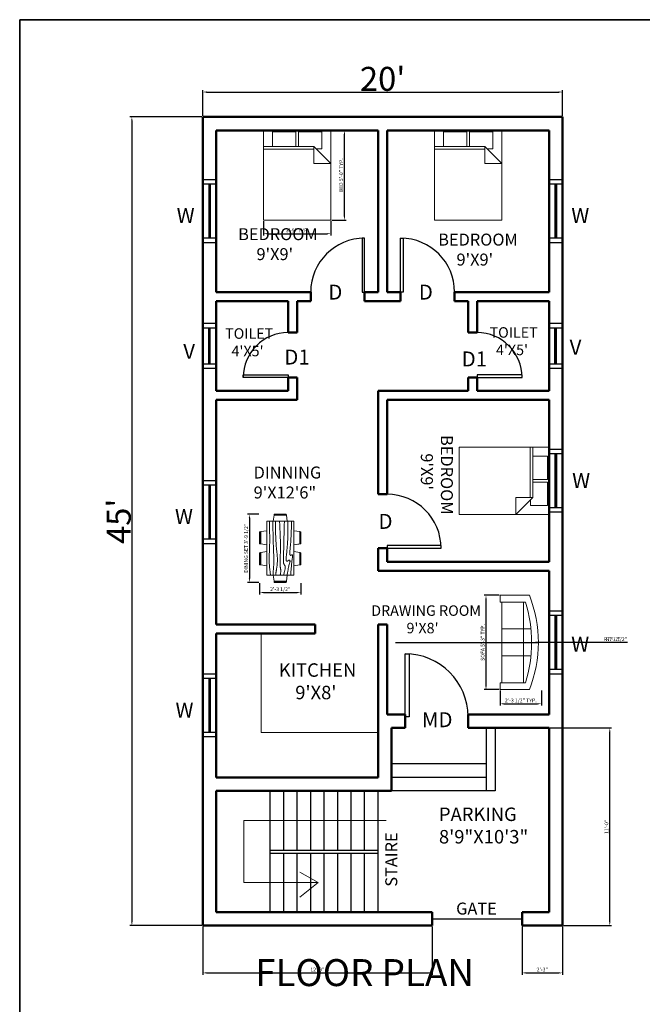
# Model space of a CAD drawing. Units: inches. Extents: x 2150 to 10686, y 1035 to 5077.
# Tile 11 of 12: x 9808 to 10224, y 1433 to 2091. Entities that reach past the tile are written whole.
import ezdxf

# ---------------------------------------------------------------- set-up
doc = ezdxf.new("R2010")
doc.units = ezdxf.units.IN
for name, color, linetype, lineweight in [('A-ANNO-DIMS', 2, 'Continuous', 18), ('A-ANNO-IDEN', 2, 'Continuous', 18), ('A-ANNO-SYMB', 3, 'Continuous', 18), ('A-ANNO-TITL', 3, 'Continuous', 35), ('A-ANNO-TTLB', 7, 'Continuous', 35), ('A-AREA-IDEN', 7, 'Continuous', 18), ('A-DOOR', 4, 'Continuous', 25), ('A-FLOR-FIXT', 9, 'Continuous', 18), ('A-FLOR-STRS', 4, 'Continuous', 25), ('A-FURN', 8, 'Continuous', 18), ('A-GLAZ', 30, 'Continuous', 25), ('A-WALL', 18, 'Continuous', 50)]:
    doc.layers.add(name, color=color, linetype=linetype, lineweight=lineweight)
doc.styles.get("Standard").update_dxf_attribs({"font": 'arial.ttf'})
doc.dimstyles.new('ISO-25', dxfattribs={"dimtxt": 2.5, "dimasz": 2.5, "dimexe": 1.25, "dimexo": 0.625, "dimtad": 1, "dimdec": 0, "dimlunit": 3, "dimtxsty": 'Standard', "dimcen": 2.5, "dimadec": 0, "dimazin": 0, "dimtfac": 1, "dimtdec": 0, "dimtmove": 0, "dimatfit": 3, "dimfxl": 1, "dimarcsym": 0})

# ---------------------------------------------------------------- blocks, each defined once
blk = doc.blocks.new('*U8')
for p, q in [((0, 0), (0, -6)), ((36, 0), (36, -6))]:
    blk.add_line(p, q)
blk.add_lwpolyline([(0, 0), (0, 36), (1.75, 36), (1.75, 0)], close=True)
blk.add_arc((0, 0), 36, 0, 90)
blk = doc.blocks.new('*U9')
for p, q in [((0, 0), (0, -6)), ((-36, 0), (-36, -6))]:
    blk.add_line(p, q)
blk.add_lwpolyline([(0, 0), (0, 36), (-1.75, 36), (-1.75, 0)], close=True)
blk.add_arc((0, 0), 36, 90, 180)
blk = doc.blocks.new('*U10')
for p, q in [((-30, 0), (-30, -6)), ((0, 0), (0, -6))]:
    blk.add_line(p, q)
blk.add_lwpolyline([(0, 0), (0, 30), (-1.75, 30), (-1.75, 0)], close=True)
blk.add_arc((0, 0), 30, 90, 180)
blk = doc.blocks.new('*U14')
for p, q in [((-30, 0), (-30, 6)), ((0, 0), (0, 6))]:
    blk.add_line(p, q)
blk.add_lwpolyline([(0, 0), (0, -30), (-1.75, -30), (-1.75, 0)], close=True)
blk.add_arc((0, 0), 30, 180, 270)
blk = doc.blocks.new('*U15')
for p, q in [((0, 0), (0, -5)), ((28, 0), (28, -5))]:
    blk.add_line(p, q)
blk.add_lwpolyline([(0, 0), (0, 28), (1.75, 28), (1.75, 0)], close=True)
blk.add_arc((0, 0), 28, 0, 90)
blk = doc.blocks.new('Bed - Queen')
for p, q in [((0, -80.00003), (0, 0)), ((0, 0), (59.99999, 0)), ((59.99999, 0), (59.99999, -80.00003)), ((7.99999, -1.2), (28.79998, -1.2)), ((7.99999, -14.4), (7.99999, -1.2)), ((28.79998, -1.2), (28.79998, -14.4)), ((31.19999, -1.2), (51.99999, -1.2)), ((31.19999, -14.4), (31.19999, -1.2)), ((51.99999, -1.2), (51.99999, -16.4)), ((0, -14.4), (44.8, -14.4)), ((44.8, -16.8), (0, -16.8)), ((59.99999, -29.6), (44.8, -14.4)), ((44.8, -14.4), (44.8, -29.6)), ((51.99999, -16.4), (46.79936, -16.4)), ((44.8, -29.6), (59.99999, -29.6)), ((59.99999, -80.00003), (0, -80.00003))]:
    blk.add_line(p, q)
blk = doc.blocks.new('Sofa - Roundback 7 ft.')
for p, q in [((-12.00002, -32.4421), (-12.00003, -6.5971)), ((11.99997, -32.4421), (11.99998, -6.5971)), ((-36.000027, -34), (-36.000027, -11.4696)), ((-35.999844, -13.3819), (35.9998, -13.3819)), ((35.99998, -34), (35.99998, -11.4696)), ((-36.000027, -32.4421), (35.99998, -32.4421))]:
    blk.add_line(p, q)
for points in [[(-36.000027, -34), (-42.000027, -34), (-42.000027, -8)], [(41.99998, -8), (41.99998, -34), (35.99998, -34)]]:
    blk.add_lwpolyline(points)
for centre, radius, start, end in [((0, -114.25), 114.25, 68.43141, 111.5686), ((-0.00001, -127.1968), 121.1968, 72.72033, 107.2797)]:
    blk.add_arc(centre, radius, start, end)
blk = doc.blocks.new('Dining Set - 36 x 72 in.')
for p, q in [((-22, 27.5), (-22.1562, 26.50042)), ((-5.8416, 26.5), (-22.1534, 26.5)), ((-22, 27.5), (-6, 27.5)), ((-5.14035, 21.99844), (-6, 27.5)), ((6, 27.5), (5.8438, 26.50042)), ((22.1584, 26.5), (5.8466, 26.5)), ((6, 27.5), (22, 27.5)), ((22.1563, 26.49966), (22, 27.5)), ((36, 18), (-36, 18)), ((-36, 18), (-36, -18)), ((-22.2343, 26.00059), (-23.4847, 17.99762)), ((-22.2304, 26), (-5.7608, 26)), ((-4.5152, 17.99762), (-5.7655, 25.99926)), ((5.7657, 26.00059), (4.5153, 17.99762)), ((5.7696, 26), (22.2392, 26)), ((23.4848, 17.99762), (22.2345, 25.99926)), ((36, -18), (36, 18)), ((-45.5, 8), (-44.5004, 8.15617)), ((-45.5, 8), (-45.5, -8)), ((-44.5, -8.15843), (-44.5, 8.15338)), ((-44.0006, 8.23428), (-35.9976, 9.48474)), ((-44, 8.23041), (-44, -8.23915)), ((44.0006, 8.23428), (35.9976, 9.48474)), ((44, 8.23041), (44, -8.23915)), ((44.5, -8.15843), (44.5, 8.15338)), ((45.5, 8), (44.5005, 8.15617)), ((45.5, 8), (45.5, -8)), ((-44.4997, -8.15631), (-45.5, -8)), ((-35.9976, -9.48476), (-43.9993, -8.2345)), ((35.9976, -9.48476), (43.9993, -8.2345)), ((44.4997, -8.15631), (45.5, -8)), ((-36, -18), (36, -18)), ((-22.2343, -26.0006), (-23.4847, -17.99762)), ((-22.2304, -26), (-5.7608, -26)), ((-4.5152, -17.99762), (-5.7655, -25.99928)), ((5.7657, -26.0006), (4.5153, -17.99762)), ((5.7696, -26), (22.2392, -26)), ((23.4848, -17.99762), (22.2345, -25.99928)), ((-22, -27.5), (-22.1562, -26.50044)), ((-5.8416, -26.5), (-22.1534, -26.5)), ((-22, -27.5), (-6, -27.5)), ((-5.8437, -26.49967), (-6, -27.5)), ((6, -27.5), (5.8438, -26.50044)), ((22.1584, -26.5), (5.8466, -26.5)), ((6, -27.5), (22, -27.5)), ((22.1563, -26.49967), (22, -27.5))]:
    blk.add_line(p, q)
for points in [[(-36, 15), (-31.1772, 14.97754), (-26.8079, 14.91406), (-22.8538, 14.81543), (-19.276, 14.6875), (-16.0362, 14.53613), (-13.0957, 14.36718), (-10.4159, 14.18652), (-7.9583, 14), (-5.6904, 13.81315), (-3.6035, 13.63021), (-1.6954, 13.45508), (0.0365, 13.29166), (1.5945, 13.14388), (2.9811, 13.01562), (4.1988, 12.9108), (5.25, 12.83333), (6.1393, 12.78613), (6.8802, 12.76823), (7.4883, 12.77767), (7.9792, 12.8125), (8.3685, 12.87077), (8.6719, 12.95052), (8.9049, 13.0498), (9.0833, 13.16666), (9.2205, 13.29899), (9.3216, 13.44401), (9.3895, 13.59879), (9.4271, 13.76041), (9.4373, 13.92594), (9.4232, 14.09245), (9.3875, 14.257), (9.3333, 14.41666), (9.2638, 14.56917), (9.1836, 14.71484), (9.0975, 14.85465), (9.0104, 14.98958), (8.9272, 15.1206), (8.8529, 15.2487), (8.7922, 15.37483), (8.75, 15.5), (8.7305, 15.62467), (8.7344, 15.74739), (8.7617, 15.86621), (8.8125, 15.97916), (8.8867, 16.08431), (8.9844, 16.17968), (9.1055, 16.26334), (9.25, 16.33333), (9.4189, 16.38802), (9.6172, 16.42708), (9.8506, 16.45052), (10.125, 16.45833), (10.4463, 16.45052), (10.8203, 16.42708), (11.2529, 16.38802), (11.75, 16.33333), (12.3184, 16.26318), (12.9694, 16.17838), (13.7151, 16.07991), (14.5677, 15.96875), (15.5395, 15.84586), (16.6426, 15.71224), (17.8893, 15.56884), (19.2917, 15.41666), (20.859, 15.25667), (22.5879, 15.08984), (24.4721, 14.91715), (26.5052, 14.73958), (28.6809, 14.5581), (30.9929, 14.3737), (33.4347, 14.18733), (36, 14)], [(-36, 10), (-28.9766, 10.14274), (-23.1725, 10.20442), (-18.4241, 10.19775), (-14.5677, 10.13541), (-11.4399, 10.03011), (-8.877, 9.89453), (-6.7154, 9.74137), (-4.7917, 9.58333), (-2.9698, 9.43082), (-1.2246, 9.28515), (0.4415, 9.14534), (2.026, 9.01041), (3.5266, 8.87939), (4.9408, 8.7513), (6.266, 8.62516), (7.5, 8.5), (8.6411, 8.37549), (9.6914, 8.2539), (10.6538, 8.13818), (11.5312, 8.03125), (12.3267, 7.93603), (13.043, 7.85547), (13.6831, 7.79248), (14.25, 7.75), (14.7471, 7.7303), (15.1797, 7.73307), (15.5537, 7.75732), (15.875, 7.80208), (16.1494, 7.86637), (16.3828, 7.94922), (16.5811, 8.04964), (16.75, 8.16666), (16.8944, 8.29915), (17.0143, 8.44531), (17.1089, 8.60319), (17.1771, 8.77083), (17.218, 8.94629), (17.2305, 9.1276), (17.2137, 9.31282), (17.1667, 9.5), (17.0895, 9.6875), (16.987, 9.875), (16.8649, 10.0625), (16.7292, 10.25), (16.5856, 10.4375), (16.4401, 10.625), (16.2985, 10.8125), (16.1667, 11), (16.05, 11.18733), (15.9518, 11.3737), (15.8752, 11.5581), (15.8229, 11.73958), (15.798, 11.91715), (15.8034, 12.08984), (15.842, 12.25667), (15.9167, 12.41666), (16.0295, 12.56836), (16.1784, 12.70833), (16.3605, 12.83268), (16.5729, 12.9375), (16.8127, 13.01888), (17.0768, 13.07291), (17.3625, 13.0957), (17.6667, 13.08333), (17.9894, 13.03312), (18.3418, 12.94726), (18.7382, 12.82918), (19.1927, 12.68229), (19.7195, 12.51001), (20.3327, 12.31575), (21.0465, 12.10294), (21.875, 11.875), (22.8357, 11.63354), (23.959, 11.37304), (25.2786, 11.08618), (26.8282, 10.76562), (28.6414, 10.40405), (30.752, 9.99414), (33.1936, 9.52856), (36, 9)], [(-36, 5.5), (-30.7157, 5.3348), (-26.069, 5.20963), (-21.9946, 5.11767), (-18.4271, 5.05208), (-15.3009, 5.00602), (-12.5508, 4.97265), (-10.1112, 4.94515), (-7.9167, 4.91666), (-5.909, 4.88167), (-4.0586, 4.83984), (-2.3429, 4.79215), (-0.7396, 4.73958), (0.7739, 4.6831), (2.22, 4.6237), (3.6213, 4.56233), (5, 4.5), (6.373, 4.43782), (7.7344, 4.3776), (9.0723, 4.32129), (10.375, 4.27083), (11.6309, 4.22819), (12.8281, 4.19531), (13.9551, 4.17415), (15, 4.16666), (15.954, 4.17448), (16.819, 4.19791), (17.6001, 4.23698), (18.3021, 4.29166), (18.9299, 4.36198), (19.4883, 4.44791), (19.9823, 4.54948), (20.4167, 4.66666), (20.7969, 4.79899), (21.1302, 4.94401), (21.4245, 5.09879), (21.6875, 5.26041), (21.9271, 5.42594), (22.1511, 5.59245), (22.3672, 5.757), (22.5834, 5.91666), (22.8065, 6.06868), (23.0404, 6.21093), (23.2879, 6.34147), (23.5521, 6.45833), (23.8358, 6.55957), (24.142, 6.64323), (24.4735, 6.70735), (24.8334, 6.75), (25.2235, 6.76969), (25.642, 6.76692), (26.0858, 6.74267), (26.5521, 6.69791), (27.0379, 6.63362), (27.5404, 6.55078), (28.0565, 6.45036), (28.5834, 6.33333), (29.1242, 6.19987), (29.7071, 6.04687), (30.3661, 5.87044), (31.1354, 5.66666), (32.0493, 5.43164), (33.142, 5.16146), (34.4475, 4.85221), (36, 4.5)], [(-36, -1), (-30.7915, -0.6591), (-26.0195, -0.38216), (-21.6519, -0.16284), (-17.6563, 0.00521), (-14.0005, 0.12833), (-10.6523, 0.21289), (-7.5796, 0.26522), (-4.75, 0.29166), (-2.134, 0.29793), (0.2878, 0.28711), (2.5317, 0.26163), (4.6146, 0.22396), (6.5529, 0.17651), (8.3633, 0.12174), (10.0623, 0.06209), (11.6667, 0), (13.1899, -0.06201), (14.6341, -0.1211), (15.9982, -0.17432), (17.2813, -0.21875), (18.4823, -0.25147), (19.6003, -0.26953), (20.6343, -0.27002), (21.5834, -0.25), (22.4481, -0.20768), (23.2357, -0.14584), (23.9549, -0.06836), (24.6146, 0.02083), (25.2235, 0.11784), (25.7904, 0.21875), (26.3241, 0.31966), (26.8334, 0.41666), (27.3265, 0.50618), (27.8099, 0.58593), (28.2894, 0.65397), (28.7709, 0.70833), (29.2601, 0.74707), (29.763, 0.76823), (30.2855, 0.76985), (30.8334, 0.75), (31.4088, 0.70784), (31.9994, 0.64713), (32.589, 0.57275), (33.1615, 0.48958), (33.7008, 0.4025), (34.1908, 0.3164), (34.6153, 0.23616), (34.9584, 0.16666), (35.2099, 0.11165), (35.3848, 0.07031), (35.504, 0.04069), (35.5886, 0.02083), (35.6594, 0.00879), (35.7377, 0.0026), (35.8442, 0.00032), (36, 0)], [(-36, -6.5), (-27.1843, -6.31267), (-20.084, -6.1263), (-14.469, -5.9419), (-10.1094, -5.76042), (-6.7752, -5.58285), (-4.2363, -5.41016), (-2.2629, -5.24333), (-0.625, -5.08334), (0.8708, -4.93099), (2.2715, -4.78646), (3.5872, -4.64974), (4.8281, -4.52084), (6.0046, -4.39974), (7.127, -4.28646), (8.2053, -4.18099), (9.25, -4.08334), (10.2705, -3.99382), (11.2734, -3.91407), (12.2647, -3.84603), (13.25, -3.79167), (14.2354, -3.75293), (15.2266, -3.73177), (16.2295, -3.73015), (17.25, -3.75), (18.2912, -3.79248), (19.3451, -3.85547), (20.4009, -3.93604), (21.4479, -4.03125), (22.4754, -4.13819), (23.4727, -4.25391), (24.4289, -4.37549), (25.3334, -4.5), (26.1785, -4.62492), (26.9694, -4.74935), (27.7145, -4.87281), (28.4219, -4.99479), (29.1, -5.11483), (29.7572, -5.23242), (30.4016, -5.34709), (31.0417, -5.45834), (31.6837, -5.56437), (32.3262, -5.65821), (32.9658, -5.73153), (33.599, -5.77604), (34.2224, -5.78345), (34.8327, -5.74545), (35.4264, -5.65373), (36, -5.5)], [(-36, -10), (-26.4022, -9.81299), (-18.4675, -9.62891), (-11.9839, -9.45069), (-6.7396, -9.28125), (-2.5226, -9.12354), (0.8789, -8.98047), (3.6769, -8.85498), (6.0833, -8.75), (8.2767, -8.66765), (10.3021, -8.60677), (12.1712, -8.56543), (13.8958, -8.54167), (15.4876, -8.53353), (16.9583, -8.53907), (18.3197, -8.55632), (19.5834, -8.58334), (20.7616, -8.61841), (21.8685, -8.66081), (22.9188, -8.71004), (23.9271, -8.76563), (24.9081, -8.82707), (25.8763, -8.89388), (26.8465, -8.96558), (27.8334, -9.04167), (28.8474, -9.12118), (29.8828, -9.20117), (30.93, -9.27824), (31.9792, -9.34896), (33.0205, -9.40991), (34.0443, -9.45768), (35.0407, -9.48885), (36, -9.5)], [(-36, -14.5), (-30.0881, -14.33513), (-25.0332, -14.21224), (-20.7312, -14.12647), (-17.0781, -14.07292), (-13.97, -14.04671), (-11.3027, -14.04297), (-8.9724, -14.05681), (-6.875, -14.08334), (-4.9224, -14.11833), (-3.0905, -14.16016), (-1.3709, -14.20785), (0.2448, -14.26042), (1.7647, -14.3169), (3.1973, -14.3763), (4.5507, -14.43767), (5.8333, -14.5), (7.0554, -14.5621), (8.235, -14.62175), (9.3922, -14.67652), (10.5469, -14.72396), (11.7192, -14.76164), (12.929, -14.78711), (14.1965, -14.79794), (15.5417, -14.79167), (16.9933, -14.76424), (18.6152, -14.70508), (20.4804, -14.60197), (22.6615, -14.44271), (25.2312, -14.21509), (28.2624, -13.9069), (31.8277, -13.50594), (36, -13)]]:
    blk.add_lwpolyline(points)
blk = doc.blocks.new('*D16')
at = {"layer": 'A-ANNO-DIMS', "color": 0, "lineweight": -2, "transparency": 16777216}
for p, q in [((9930.51, 2026.59), (9930.51, 2043.8)), ((9933.01, 2042.55), (10168.01, 2042.55)), ((10170.51, 2026.59), (10170.51, 2043.8))]:
    blk.add_line(p, q, dxfattribs=at)
at = {"layer": 'A-ANNO-DIMS', "color": 0, "transparency": 16777216}
for points in [[(9933.01, 2042.97), (9933.01, 2042.14), (9930.51, 2042.55)], [(10168.01, 2042.97), (10168.01, 2042.14), (10170.51, 2042.55)]]:
    blk.add_solid(points, dxfattribs=at)
at = {"layer": 'Defpoints', "color": 0, "transparency": 16777216}
for p in [(10170.51, 2042.55), (9930.51, 2025.96), (10170.51, 2025.96)]:
    blk.add_point(p, dxfattribs=at)
at = {"layer": 'A-ANNO-DIMS', "color": 0, "transparency": 16777216, "insert": (10050.51, 2051.35), "char_height": 2.5, "attachment_point": 5}
blk.add_mtext("{\\H6.4x;20'}", dxfattribs=at)
blk = doc.blocks.new('*D17')
at = {"layer": 'A-ANNO-DIMS', "color": 0, "lineweight": -2, "transparency": 16777216}
for p, q in [((9929.88, 2025.96), (9881.93, 2025.96)), ((9883.18, 2023.46), (9883.18, 1488.46)), ((9929.88, 1485.96), (9881.93, 1485.96))]:
    blk.add_line(p, q, dxfattribs=at)
at = {"layer": 'A-ANNO-DIMS', "color": 0, "transparency": 16777216}
for points in [[(9882.76, 2023.46), (9883.6, 2023.46), (9883.18, 2025.96)], [(9882.76, 1488.46), (9883.6, 1488.46), (9883.18, 1485.96)]]:
    blk.add_solid(points, dxfattribs=at)
at = {"layer": 'Defpoints', "color": 0, "transparency": 16777216}
for p in [(9930.51, 2025.96), (9883.18, 1485.96), (9930.51, 1485.96)]:
    blk.add_point(p, dxfattribs=at)
at = {"layer": 'A-ANNO-DIMS', "color": 0, "transparency": 16777216, "insert": (9874.42, 1755.96), "char_height": 2.5, "attachment_point": 5, "rotation": 90}
blk.add_mtext("{\\H6.4x;45'}", dxfattribs=at)
blk = doc.blocks.new('WINDOW-36IN')
for p, q in [((9, 42), (0, 42)), ((9, 39), (0, 39)), ((4, 39), (4, 3)), ((4.5, 39), (4.5, 3)), ((5, 39), (5, 3)), ((9, 3), (0, 3)), ((9, 0), (0, 0))]:
    blk.add_line(p, q)
blk = doc.blocks.new('VENT-24IN')
for p, q in [((0, 30), (9, 30)), ((0, 27), (9, 27)), ((4, 27), (4, 3)), ((4.5, 27), (4.5, 3)), ((5, 27), (5, 3)), ((0, 3), (9, 3)), ((0, 0), (9, 0))]:
    blk.add_line(p, q)
blk = doc.blocks.new('*D42')
at = {"layer": 'A-ANNO-DIMS', "color": 0, "lineweight": -2, "transparency": 16777216}
for p, q in [((10016.63, 2016.96), (10026.26, 2016.96)), ((10025.01, 1959.46), (10025.01, 2014.46)), ((10016.63, 1956.96), (10026.26, 1956.96))]:
    blk.add_line(p, q, dxfattribs=at)
at = {"layer": 'A-ANNO-DIMS', "color": 0, "transparency": 16777216}
for points in [[(10024.59, 2014.46), (10025.42, 2014.46), (10025.01, 2016.96)], [(10024.59, 1959.46), (10025.42, 1959.46), (10025.01, 1956.96)]]:
    blk.add_solid(points, dxfattribs=at)
at = {"layer": 'Defpoints', "color": 0, "transparency": 16777216}
for p in [(10016.01, 2016.96), (10025.01, 2016.96), (10016.01, 1956.96)]:
    blk.add_point(p, dxfattribs=at)
at = {"layer": 'A-ANNO-DIMS', "color": 0, "transparency": 16777216, "insert": (10023.11, 1986.96), "char_height": 2.5, "attachment_point": 5, "rotation": 90}
blk.add_mtext('BED 5\'-0" TYP.', dxfattribs=at)
blk = doc.blocks.new('*D43')
at = {"layer": 'A-ANNO-DIMS', "color": 0, "lineweight": -2, "transparency": 16777216}
for p, q in [((9971.01, 1956.34), (9971.01, 1946.71)), ((10016.01, 1956.34), (10016.01, 1946.71)), ((9973.51, 1947.96), (10013.51, 1947.96))]:
    blk.add_line(p, q, dxfattribs=at)
at = {"layer": 'A-ANNO-DIMS', "color": 0, "transparency": 16777216}
for points in [[(9973.51, 1948.38), (9973.51, 1947.55), (9971.01, 1947.96)], [(10013.51, 1948.38), (10013.51, 1947.55), (10016.01, 1947.96)]]:
    blk.add_solid(points, dxfattribs=at)
at = {"layer": 'Defpoints', "color": 0, "transparency": 16777216}
for p in [(9971.01, 1956.96), (10016.01, 1956.96), (10016.01, 1947.96)]:
    blk.add_point(p, dxfattribs=at)
at = {"layer": 'A-ANNO-DIMS', "color": 0, "transparency": 16777216, "insert": (9993.51, 1949.87), "char_height": 2.5, "attachment_point": 5}
blk.add_mtext('3\'-9" TYP.', dxfattribs=at)
blk = doc.blocks.new('*D50')
at = {"layer": 'A-ANNO-DIMS', "color": 0, "lineweight": -2, "transparency": 16777216}
for p, q in [((10128.3, 1706.54), (10118.22, 1706.54)), ((10119.47, 1704.04), (10119.47, 1646.04)), ((10128.3, 1643.54), (10118.22, 1643.54))]:
    blk.add_line(p, q, dxfattribs=at)
at = {"layer": 'A-ANNO-DIMS', "color": 0, "transparency": 16777216}
for points in [[(10119.06, 1704.04), (10119.89, 1704.04), (10119.47, 1706.54)], [(10119.06, 1646.04), (10119.89, 1646.04), (10119.47, 1643.54)]]:
    blk.add_solid(points, dxfattribs=at)
at = {"layer": 'Defpoints', "color": 0, "transparency": 16777216}
for p in [(10128.92, 1706.54), (10119.47, 1643.54), (10128.92, 1643.54)]:
    blk.add_point(p, dxfattribs=at)
at = {"layer": 'A-ANNO-DIMS', "color": 0, "transparency": 16777216, "insert": (10117.56, 1675.04), "char_height": 2.5, "attachment_point": 5, "rotation": 90}
blk.add_mtext('SOFA 5\'-3" TYP.', dxfattribs=at)
blk = doc.blocks.new('*D51')
at = {"layer": 'A-ANNO-DIMS', "color": 0, "lineweight": -2, "transparency": 16777216}
for p, q in [((10128.92, 1642.91), (10128.92, 1632.84)), ((10156.42, 1642.91), (10156.42, 1632.84)), ((10131.42, 1634.09), (10153.92, 1634.09))]:
    blk.add_line(p, q, dxfattribs=at)
at = {"layer": 'A-ANNO-DIMS', "color": 0, "transparency": 16777216}
for points in [[(10131.42, 1634.5), (10131.42, 1633.67), (10128.92, 1634.09)], [(10153.92, 1634.5), (10153.92, 1633.67), (10156.42, 1634.09)]]:
    blk.add_solid(points, dxfattribs=at)
at = {"layer": 'Defpoints', "color": 0, "transparency": 16777216}
for p in [(10128.92, 1643.54), (10156.42, 1643.54), (10156.42, 1634.09)]:
    blk.add_point(p, dxfattribs=at)
at = {"layer": 'A-ANNO-DIMS', "color": 0, "transparency": 16777216, "insert": (10142.67, 1636.01), "char_height": 2.5, "attachment_point": 5}
blk.add_mtext('2\'-3 1/2" TYP.', dxfattribs=at)
blk = doc.blocks.new('*D58')
at = {"layer": 'A-ANNO-DIMS', "color": 0, "lineweight": -2, "transparency": 16777216}
for p, q in [((9967.8, 1760.67), (9960.35, 1760.67)), ((9961.6, 1758.17), (9961.6, 1717.67)), ((9967.8, 1715.17), (9960.35, 1715.17))]:
    blk.add_line(p, q, dxfattribs=at)
at = {"layer": 'A-ANNO-DIMS', "color": 0, "transparency": 16777216}
for points in [[(9961.18, 1758.17), (9962.01, 1758.17), (9961.6, 1760.67)], [(9961.18, 1717.67), (9962.01, 1717.67), (9961.6, 1715.17)]]:
    blk.add_solid(points, dxfattribs=at)
at = {"layer": 'Defpoints', "color": 0, "transparency": 16777216}
for p in [(9968.42, 1760.67), (9961.6, 1715.17), (9968.42, 1715.17)]:
    blk.add_point(p, dxfattribs=at)
at = {"layer": 'A-ANNO-DIMS', "color": 0, "transparency": 16777216, "insert": (9959.68, 1737.92), "char_height": 2.5, "attachment_point": 5, "rotation": 90}
blk.add_mtext('DINING SET 3\'-9 1/2"', dxfattribs=at)
blk = doc.blocks.new('*D59')
at = {"layer": 'A-ANNO-DIMS', "color": 0, "lineweight": -2, "transparency": 16777216}
for p, q in [((9968.42, 1714.55), (9968.42, 1707.1)), ((9995.92, 1714.55), (9995.92, 1707.1)), ((9970.92, 1708.35), (9993.42, 1708.35))]:
    blk.add_line(p, q, dxfattribs=at)
at = {"layer": 'A-ANNO-DIMS', "color": 0, "transparency": 16777216}
for points in [[(9970.92, 1708.76), (9970.92, 1707.93), (9968.42, 1708.35)], [(9993.42, 1708.76), (9993.42, 1707.93), (9995.92, 1708.35)]]:
    blk.add_solid(points, dxfattribs=at)
at = {"layer": 'Defpoints', "color": 0, "transparency": 16777216}
for p in [(9968.42, 1715.17), (9995.92, 1715.17), (9995.92, 1708.35)]:
    blk.add_point(p, dxfattribs=at)
at = {"layer": 'A-ANNO-DIMS', "color": 0, "transparency": 16777216, "insert": (9982.17, 1710.26), "char_height": 2.5, "attachment_point": 5}
blk.add_mtext('2\'-3 1/2"', dxfattribs=at)
blk = doc.blocks.new('*D141')
at = {"layer": 'A-ANNO-DIMS', "color": 0, "lineweight": -2, "transparency": 16777216}
for p, q in [((9930.51, 1485.34), (9930.51, 1453.16)), ((10083.51, 1485.34), (10083.51, 1453.16)), ((9933.01, 1454.41), (10081.01, 1454.41))]:
    blk.add_line(p, q, dxfattribs=at)
at = {"layer": 'A-ANNO-DIMS', "color": 0, "transparency": 16777216}
for points in [[(9933.01, 1454.83), (9933.01, 1454), (9930.51, 1454.41)], [(10081.01, 1454.83), (10081.01, 1454), (10083.51, 1454.41)]]:
    blk.add_solid(points, dxfattribs=at)
at = {"layer": 'Defpoints', "color": 0, "transparency": 16777216}
for p in [(9930.51, 1485.96), (10083.51, 1485.96), (10083.51, 1454.41)]:
    blk.add_point(p, dxfattribs=at)
at = {"layer": 'A-ANNO-DIMS', "color": 0, "transparency": 16777216, "insert": (10007.01, 1456.32), "char_height": 2.5, "attachment_point": 5}
blk.add_mtext('12\'-9"', dxfattribs=at)
blk = doc.blocks.new('*D142')
at = {"layer": 'A-ANNO-DIMS', "color": 0, "lineweight": -2, "transparency": 16777216}
for p, q in [((10143.51, 1485.34), (10143.51, 1453.16)), ((10170.51, 1485.34), (10170.51, 1453.16)), ((10146.01, 1454.41), (10168.01, 1454.41))]:
    blk.add_line(p, q, dxfattribs=at)
at = {"layer": 'A-ANNO-DIMS', "color": 0, "transparency": 16777216}
for points in [[(10146.01, 1454.83), (10146.01, 1454), (10143.51, 1454.41)], [(10168.01, 1454.83), (10168.01, 1454), (10170.51, 1454.41)]]:
    blk.add_solid(points, dxfattribs=at)
at = {"layer": 'Defpoints', "color": 0, "transparency": 16777216}
for p in [(10143.51, 1485.96), (10170.51, 1485.96), (10170.51, 1454.41)]:
    blk.add_point(p, dxfattribs=at)
at = {"layer": 'A-ANNO-DIMS', "color": 0, "transparency": 16777216, "insert": (10157.01, 1456.32), "char_height": 2.5, "attachment_point": 5}
blk.add_mtext('2\'-3"', dxfattribs=at)
blk = doc.blocks.new('*D143')
at = {"layer": 'A-ANNO-DIMS', "color": 0, "lineweight": -2, "transparency": 16777216}
for p, q in [((10162.13, 1617.96), (10203.31, 1617.96)), ((10202.06, 1488.46), (10202.06, 1615.46)), ((10171.13, 1485.96), (10203.31, 1485.96))]:
    blk.add_line(p, q, dxfattribs=at)
at = {"layer": 'A-ANNO-DIMS', "color": 0, "transparency": 16777216}
for points in [[(10201.64, 1615.46), (10202.47, 1615.46), (10202.06, 1617.96)], [(10201.64, 1488.46), (10202.47, 1488.46), (10202.06, 1485.96)]]:
    blk.add_solid(points, dxfattribs=at)
at = {"layer": 'Defpoints', "color": 0, "transparency": 16777216}
for p in [(10161.51, 1617.96), (10202.06, 1617.96), (10170.51, 1485.96)]:
    blk.add_point(p, dxfattribs=at)
at = {"layer": 'A-ANNO-DIMS', "color": 0, "transparency": 16777216, "insert": (10200.16, 1551.96), "char_height": 2.5, "attachment_point": 5, "rotation": 90}
blk.add_mtext('11\'-0"', dxfattribs=at)
blk = doc.blocks.new('*D153')
at = {"layer": 'A-ANNO-DIMS', "color": 0, "lineweight": -2, "transparency": 16777216}
for p, q in [((10059.03, 1675.04), (10149.92, 1675.04)), ((10209.61, 1675.04), (10152.42, 1675.04))]:
    blk.add_line(p, q, dxfattribs=at)
at = {"layer": 'A-ANNO-DIMS', "color": 0, "transparency": 16777216}
blk.add_solid([(10152.42, 1675.45), (10152.42, 1674.62), (10149.92, 1675.04)], dxfattribs=at)
at = {"layer": 'Defpoints', "color": 0, "transparency": 16777216}
for p in [(10059.03, 1675.04), (10149.92, 1675.04)]:
    blk.add_point(p, dxfattribs=at)
at = {"layer": 'A-ANNO-DIMS', "color": 0, "transparency": 16777216, "insert": (10204.46, 1676.91), "char_height": 2.5, "attachment_point": 5, "rotation": 359.99989}
blk.add_mtext('R7\'-7"', dxfattribs=at)
blk = doc.blocks.new('*D154')
at = {"layer": 'A-ANNO-DIMS', "color": 0, "lineweight": -2, "transparency": 16777216}
for p, q in [((10068.74, 1675.04), (10154.42, 1675.04)), ((10213.89, 1675.04), (10156.92, 1675.04))]:
    blk.add_line(p, q, dxfattribs=at)
at = {"layer": 'A-ANNO-DIMS', "color": 0, "transparency": 16777216}
blk.add_solid([(10156.92, 1675.45), (10156.92, 1674.62), (10154.42, 1675.04)], dxfattribs=at)
at = {"layer": 'Defpoints', "color": 0, "transparency": 16777216}
for p in [(10068.74, 1675.04), (10154.42, 1675.04)]:
    blk.add_point(p, dxfattribs=at)
at = {"layer": 'A-ANNO-DIMS', "color": 0, "transparency": 16777216, "insert": (10205.84, 1676.95), "char_height": 2.5, "attachment_point": 5, "rotation": 359.99989}
blk.add_mtext('R7\'-1 1/2"', dxfattribs=at)

msp = doc.modelspace()

# ---------------------------------------------------------------- linework, layer by layer
at = {"layer": 'A-ANNO-SYMB'}
for p, q in [((10052.83, 1556.21), (9957.79, 1556.21)), ((9957.79, 1556.21), (9957.79, 1514.71)), ((10007.53, 1514.71), (9995.3, 1521.56)), ((9957.79, 1514.71), (10007.53, 1514.71)), ((10007.53, 1514.71), (9995.15, 1504.92))]:
    msp.add_line(p, q, dxfattribs=at)
at = {"layer": 'A-ANNO-TTLB'}
msp.add_lwpolyline([(9808.35, 2090.85), (10686.34, 2090.85), (10686.34, 1034.91), (9808.35, 1034.91)], close=True, dxfattribs=at)
at = {"layer": 'A-DOOR'}
msp.add_line((10083.51, 1490.46), (10143.51, 1490.46), dxfattribs=at)
at = {"layer": 'A-FLOR-FIXT'}
for q in [(9969.51, 1680.96), (10047.51, 1614.96)]:
    msp.add_line((9969.51, 1614.96), q, dxfattribs=at)
at = {"layer": 'A-FLOR-STRS'}
for p, q in [((10119.51, 1617.96), (10119.51, 1575.96)), ((10125.51, 1617.96), (10125.51, 1575.96)), ((10119.51, 1593.96), (10056.51, 1593.96)), ((10119.51, 1584.96), (10056.51, 1584.96)), ((9975.51, 1494.96), (9975.51, 1575.96)), ((9984.51, 1536.46), (9984.51, 1575.96)), ((9993.51, 1536.46), (9993.51, 1575.96)), ((10002.51, 1536.46), (10002.51, 1575.96)), ((10011.51, 1536.46), (10011.51, 1575.96)), ((10020.51, 1536.46), (10020.51, 1575.96)), ((10029.51, 1536.46), (10029.51, 1575.96)), ((10038.51, 1536.46), (10038.51, 1575.96)), ((10047.51, 1494.96), (10047.51, 1575.96)), ((10125.51, 1575.96), (10056.51, 1575.96)), ((9975.51, 1536.46), (10047.51, 1536.46)), ((9975.51, 1534.46), (10047.51, 1534.46)), ((9984.51, 1494.96), (9984.51, 1534.46)), ((9993.51, 1494.96), (9993.51, 1534.46)), ((10002.51, 1494.96), (10002.51, 1534.46)), ((10011.51, 1494.96), (10011.51, 1534.46)), ((10020.51, 1494.96), (10020.51, 1534.46)), ((10029.51, 1494.96), (10029.51, 1534.46)), ((10038.51, 1494.96), (10038.51, 1534.46))]:
    msp.add_line(p, q, dxfattribs=at)
at = {"layer": 'A-WALL'}
for p, q in [((9930.51, 2025.96), (10170.51, 2025.96)), ((9930.51, 1485.96), (9930.51, 2025.96)), ((10170.51, 2025.96), (10170.51, 1485.96)), ((9939.51, 2016.96), (10047.51, 2016.96)), ((9939.51, 1908.96), (9939.51, 2016.96)), ((10047.51, 2016.96), (10047.51, 1908.96)), ((10053.51, 2016.96), (10053.51, 1908.96)), ((10053.51, 2016.96), (10161.51, 2016.96)), ((10161.51, 2016.96), (10161.51, 1908.96)), ((9939.51, 1908.96), (10002.51, 1908.96)), ((10002.51, 1908.96), (10002.51, 1902.96)), ((10038.51, 1908.96), (10038.51, 1902.96)), ((10038.51, 1908.96), (10047.51, 1908.96)), ((10053.51, 1908.96), (10062.51, 1908.96)), ((10062.51, 1908.96), (10062.51, 1902.96)), ((10098.51, 1908.96), (10098.51, 1902.96)), ((10098.51, 1908.96), (10161.51, 1908.96)), ((9939.51, 1902.96), (9987.51, 1902.96)), ((9939.51, 1842.96), (9939.51, 1902.96)), ((9987.51, 1881.96), (9987.51, 1902.96)), ((9993.51, 1881.96), (9993.51, 1902.96)), ((9993.51, 1902.96), (10002.51, 1902.96)), ((10038.51, 1902.96), (10062.51, 1902.96)), ((10098.51, 1902.96), (10107.51, 1902.96)), ((10107.51, 1902.96), (10107.51, 1881.96)), ((10113.51, 1902.96), (10113.51, 1881.96)), ((10113.51, 1902.96), (10161.51, 1902.96)), ((10161.51, 1902.96), (10161.51, 1842.96)), ((9987.51, 1881.96), (9993.51, 1881.96)), ((10107.51, 1881.96), (10113.51, 1881.96)), ((9987.51, 1842.96), (9987.51, 1851.96)), ((9987.51, 1851.96), (9993.51, 1851.96)), ((9993.51, 1836.96), (9993.51, 1851.96)), ((10107.51, 1851.96), (10113.51, 1851.96)), ((10107.51, 1851.96), (10107.51, 1842.96)), ((10113.51, 1851.96), (10113.51, 1842.96)), ((9939.51, 1842.96), (9987.51, 1842.96)), ((10047.51, 1842.96), (10047.51, 1773.96)), ((10047.51, 1842.96), (10107.51, 1842.96)), ((10113.51, 1842.96), (10161.51, 1842.96)), ((9939.51, 1836.96), (9993.51, 1836.96)), ((9939.51, 1686.96), (9939.51, 1836.96)), ((10053.51, 1836.96), (10053.51, 1773.96)), ((10053.51, 1836.96), (10161.51, 1836.96)), ((10161.51, 1836.96), (10161.51, 1728.96)), ((10047.51, 1773.96), (10053.51, 1773.96)), ((10047.51, 1737.96), (10053.51, 1737.96)), ((10047.51, 1737.96), (10047.51, 1722.96)), ((10053.51, 1737.96), (10053.51, 1728.96)), ((10047.51, 1722.96), (10161.51, 1722.96)), ((10053.51, 1728.96), (10161.51, 1728.96)), ((10161.51, 1722.96), (10161.51, 1626.96)), ((9939.51, 1686.96), (10005.51, 1686.96)), ((10005.51, 1680.96), (10005.51, 1686.96)), ((10047.51, 1686.96), (10053.51, 1686.96)), ((10047.51, 1686.96), (10047.51, 1584.96)), ((10053.51, 1686.96), (10053.51, 1626.96)), ((9939.51, 1584.96), (9939.51, 1680.96)), ((9939.51, 1680.96), (10005.51, 1680.96)), ((10053.51, 1626.96), (10065.51, 1626.96)), ((10065.51, 1626.96), (10065.51, 1617.96)), ((10107.51, 1626.96), (10107.51, 1617.96)), ((10107.51, 1626.96), (10161.51, 1626.96)), ((10056.51, 1617.96), (10065.51, 1617.96)), ((10056.51, 1617.96), (10056.51, 1575.96)), ((10107.51, 1617.96), (10161.51, 1617.96)), ((10161.51, 1617.96), (10161.51, 1494.96)), ((9939.51, 1584.96), (10047.51, 1584.96)), ((9939.51, 1494.96), (9939.51, 1575.96)), ((9939.51, 1575.96), (10056.51, 1575.96)), ((10083.51, 1494.96), (9939.51, 1494.96)), ((10083.51, 1494.96), (10083.51, 1485.96)), ((10161.51, 1494.96), (10143.51, 1494.96)), ((10143.51, 1494.96), (10143.51, 1485.96)), ((10083.51, 1485.96), (9930.51, 1485.96)), ((10170.51, 1485.96), (10143.51, 1485.96))]:
    msp.add_line(p, q, dxfattribs=at)

# ---------------------------------------------------------------- block references
at = {"layer": 'A-DOOR'}
for name, p in [('*U9', (10038.51, 1908.96)), ('*U8', (10062.51, 1908.96))]:
    msp.add_blockref(name, p, dxfattribs=at)
at = {"layer": 'A-DOOR', "rotation": 270}
for name, p in [('*U14', (9987.51, 1851.96)), ('*U10', (10113.51, 1851.96)), ('*U9', (10053.51, 1737.96))]:
    msp.add_blockref(name, p, dxfattribs=at)
at = {"layer": 'A-DOOR', "xscale": 1.5, "yscale": 1.5, "zscale": 1.5}
msp.add_blockref('*U15', (10065.51, 1625.46), dxfattribs=at)
at = {"layer": 'A-FURN', "xscale": 0.75, "yscale": 0.75, "zscale": 0.75}
for p in [(9971.01, 2016.96), (10085.01, 2016.96)]:
    msp.add_blockref('Bed - Queen', p, dxfattribs=at)
at = {"layer": 'A-FURN', "rotation": 270}
for name, p, xscale, yscale, zscale in [('Bed - Queen', (10161.51, 1805.46), 0.75, 0.75, 0.75), ('Dining Set - 36 x 72 in.', (9982.17, 1737.92), 0.5, 0.5, 0.5), ('Sofa - Roundback 7 ft.', (10154.42, 1675.04), 0.75, 0.75, 0.75)]:
    msp.add_blockref(name, p, dxfattribs=dict(at, xscale=xscale, yscale=yscale, zscale=zscale))
at = {"layer": 'A-GLAZ'}
for p in [(9930.51, 1941.96), (10161.51, 1941.96), (10161.51, 1761.96), (9930.51, 1740.96), (10161.51, 1653.96), (9930.51, 1611.96)]:
    msp.add_blockref('WINDOW-36IN', p, dxfattribs=at)
at = {"layer": 'A-GLAZ', "rotation": 180}
for p in [(9939.51, 1887.96), (10170.51, 1887.96)]:
    msp.add_blockref('VENT-24IN', p, dxfattribs=at)

# ---------------------------------------------------------------- texts
at = {"layer": 'A-ANNO-IDEN', "attachment_point": 1}
for s, width, insert, char_height in [('W', 356.3185, (9913.08, 1965.2), 10), ('W', 356.3185, (10176.4, 1965.15), 10), ('D', 356.3185, (10014.26, 1913.96), 10), ('D', 356.3185, (10074.64, 1913.96), 10), ('V', 356.3185, (9917.48, 1874.42), 10), ('V', 356.3185, (10175.26, 1877.17), 10), ('D1', 356.3185, (9984.91, 1870.6), 10), ('D1', 356.3185, (10103.24, 1869.33), 10), ('W', 356.3185, (10176.97, 1788.15), 10), ('W', 356.3185, (9911.95, 1764.11), 10), ('D', 356.3185, (10047.74, 1760.88), 10), ('W', 356.3185, (10176.32, 1678.85), 10), ('W', 356.3185, (9912.31, 1634.91), 10), ('MD', 356.3185, (10076.67, 1628.47), 10), ('GATE', 97.4793, (10099.55, 1501.35), 8)]:
    msp.add_mtext_dynamic_manual_height_columns(s, width=width, gutter_width=12.5, heights=[0], dxfattribs=dict(at, insert=insert, char_height=char_height))
at = {"layer": 'A-ANNO-TITL', "insert": (9965.45, 1463.6), "char_height": 18, "attachment_point": 1}
msp.add_mtext_dynamic_manual_height_columns('FLOOR PLAN', width=1484.0735, gutter_width=12.5, heights=[0], dxfattribs=at)
at = {"layer": 'A-AREA-IDEN', "attachment_point": 1}
for s, width, insert, char_height in [("BEDROOM\\P     9'X9'", 304.341, (9954.11, 1951.65), 8), ("BEDROOM\\P     9'X9'", 180.0961, (10087.58, 1948.02), 8), ("TOILET\\P  4'X5'", 141.2563, (9945.39, 1884.8), 7), ("TOILET\\P  4'X5'", 141.2563, (10121.85, 1885.53), 7), ('DINNING\\P9\'X12\'6"', 305.3587, (9964.43, 1792.5), 8), ("DRAWING ROOM\\P           9'X8'", 291.5879, (10042.9, 1699.81), 7), ("KITCHEN\\P    9'X8'", 322.616, (9981.2, 1661.11), 9), ('PARKING\\P8\'9"X10\'3"', 244.8476, (10088.07, 1564.82), 9)]:
    msp.add_mtext_dynamic_manual_height_columns(s, width=width, gutter_width=12.5, heights=[0], dxfattribs=dict(at, insert=insert, char_height=char_height))
at = {"layer": 'A-AREA-IDEN', "char_height": 8, "attachment_point": 1}
for s, width, insert, rotation in [("BEDROOM\\P     9'X9'", 180.0961, (10097.36, 1813.53), 270), ('STAIRE', 164.3588, (10052.29, 1511.97), 90)]:
    msp.add_mtext_dynamic_manual_height_columns(s, width=width, gutter_width=12.5, heights=[0], dxfattribs=dict(at, insert=insert, rotation=rotation))

# ---------------------------------------------------------------- dimensions: what is measured, and where the dimension line sits
at = {"layer": 'A-ANNO-DIMS'}
for base, p1, p2, text, override, picture, middle in [((10170.51, 2042.55), (9930.51, 2025.96), (10170.51, 2025.96), '{\\H6.4x;<>}', {"dimclrd": 0, "dimclre": 0, "dimclrt": 0}, '*D16', (10050.51, 2051.35)), ((10016.01, 1947.96), (9971.01, 1956.96), (10016.01, 1956.96), '<> TYP.', {"dimdec": 1, "dimlfac": 1, "dimrnd": 0, "dimzin": 1, "dimdsep": 46, "dimlunit": 4, "dimfrac": 2}, '*D43', (9993.51, 1949.87)), ((10156.42, 1634.09), (10128.92, 1643.54), (10156.42, 1643.54), '<> TYP.', {"dimdec": 1, "dimlfac": 1, "dimrnd": 0, "dimzin": 1, "dimdsep": 46, "dimlunit": 4, "dimfrac": 2}, '*D51', (10142.67, 1636.01))]:
    dim = msp.add_linear_dim(base=base, p1=p1, p2=p2, text=text, dimstyle='ISO-25', override=override, dxfattribs=at)
    dim.commit()
    dim.dimension.update_dxf_attribs({"geometry": picture, "text_midpoint": middle})
for base, p1, p2, angle, text, override, picture, middle in [((9883.18, 1485.96), (9930.51, 2025.96), (9930.51, 1485.96), 90, '{\\H6.4x;<>}', {"dimclrd": 0, "dimclre": 0, "dimclrt": 0}, '*D17', (9874.42, 1755.96)), ((10025.01, 2016.96), (10016.01, 1956.96), (10016.01, 2016.96), 90, 'BED <> TYP.', {"dimdec": 1, "dimlfac": 1, "dimrnd": 0, "dimzin": 1, "dimdsep": 46, "dimlunit": 4, "dimfrac": 2}, '*D42', (10023.11, 1986.96)), ((9961.6, 1715.17), (9968.42, 1760.67), (9968.42, 1715.17), 270, 'DINING SET <>', {"dimdec": 1, "dimlfac": 1, "dimrnd": 0, "dimzin": 1, "dimdsep": 46, "dimlunit": 4, "dimfrac": 2}, '*D58', (9959.68, 1737.92)), ((10119.47, 1643.54), (10128.92, 1706.54), (10128.92, 1643.54), 270, 'SOFA <> TYP.', {"dimdec": 1, "dimlfac": 1, "dimrnd": 0, "dimzin": 1, "dimdsep": 46, "dimlunit": 4, "dimfrac": 2}, '*D50', (10117.56, 1675.04))]:
    dim = msp.add_linear_dim(base=base, p1=p1, p2=p2, angle=angle, text=text, dimstyle='ISO-25', override=override, dxfattribs=at)
    dim.commit()
    dim.dimension.update_dxf_attribs({"geometry": picture, "text_midpoint": middle})
for base, p1, p2, picture, middle in [((9995.92, 1708.35), (9968.42, 1715.17), (9995.92, 1715.17), '*D59', (9982.17, 1710.26)), ((10083.51, 1454.41), (9930.51, 1485.96), (10083.51, 1485.96), '*D141', (10007.01, 1456.32)), ((10170.51, 1454.41), (10143.51, 1485.96), (10170.51, 1485.96), '*D142', (10157.01, 1456.32))]:
    dim = msp.add_linear_dim(base=base, p1=p1, p2=p2, dimstyle='ISO-25', override={"dimdec": 1, "dimlfac": 1, "dimrnd": 0, "dimzin": 1, "dimdsep": 46, "dimlunit": 4, "dimfrac": 2}, dxfattribs=at)
    dim.commit()
    dim.dimension.update_dxf_attribs({"geometry": picture, "text_midpoint": middle})
for center, mpoint, picture, middle in [((10059.03, 1675.04), (10149.92, 1675.04), '*D153', (10204.46, 1675.04)), ((10068.74, 1675.04), (10154.42, 1675.04), '*D154', (10205.84, 1675.04))]:
    dim = msp.add_radius_dim(center=center, mpoint=mpoint, dimstyle='ISO-25', override={"dimdec": 1, "dimlfac": 1, "dimrnd": 0, "dimzin": 1, "dimdsep": 46, "dimlunit": 4, "dimfrac": 2}, dxfattribs=at)
    dim.commit()
    dim.dimension.update_dxf_attribs({"geometry": picture, "text_midpoint": middle, "dimtype": 164})
dim = msp.add_linear_dim(base=(10202.06, 1617.96), p1=(10170.51, 1485.96), p2=(10161.51, 1617.96), angle=90, dimstyle='ISO-25', override={"dimdec": 1, "dimlfac": 1, "dimrnd": 0, "dimzin": 1, "dimdsep": 46, "dimlunit": 4, "dimfrac": 2}, dxfattribs=at)
dim.commit()
dim.dimension.update_dxf_attribs({"geometry": '*D143', "text_midpoint": (10200.16, 1551.96)})

doc.saveas('drawing.dxf')
